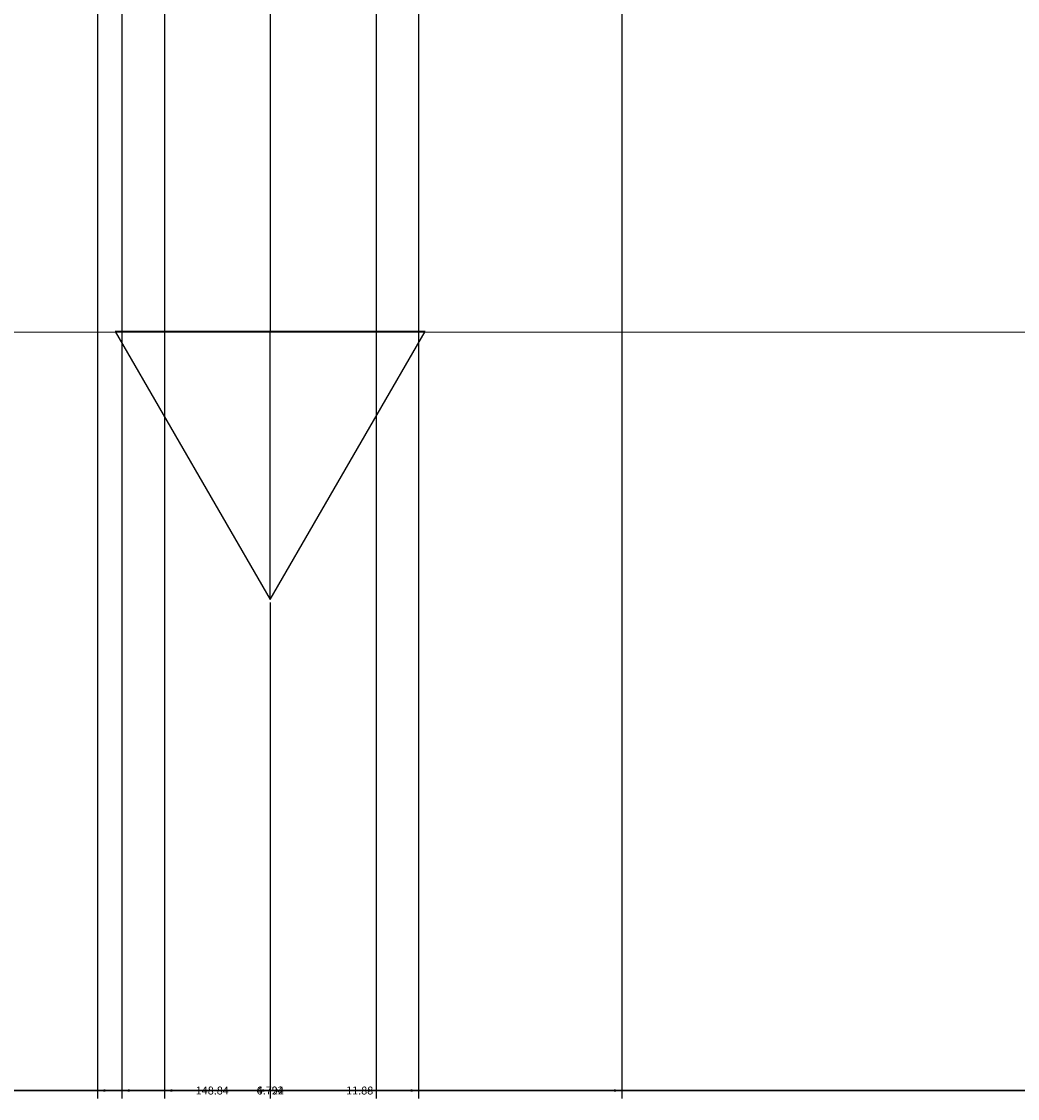
# Model space of a CAD drawing. Units: inches. Extents: x 412 to 584, y 208 to 437.
# Tile 6 of 28: x 494 to 516, y 208 to 233. Entities that reach past the tile are written whole.
import ezdxf

# ---------------------------------------------------------------- set-up
doc = ezdxf.new("R2010")
doc.units = ezdxf.units.IN
doc.header["$MEASUREMENT"] = 0
for name, color, linetype, lineweight in [('A-ANNO-DIMS', 2, 'Continuous', 18), ('E-ENCL', 8, 'Continuous', 18), ('E-POWR-EQPM', 3, 'Continuous', 25)]:
    doc.layers.add(name, color=color, linetype=linetype, lineweight=lineweight)
doc.styles.get("Standard").update_dxf_attribs({"font": 'arial.ttf'})
doc.dimstyles.get("Standard").update_dxf_attribs({"dimtxt": 0.18, "dimasz": 0.18, "dimexe": 0.18, "dimexo": 0.0625, "dimgap": 0.09, "dimtad": 0, "dimtih": 1, "dimtoh": 1, "dimdec": 4, "dimzin": 0, "dimdsep": 46, "dimtxsty": 'Standard', "dimcen": 0.09, "dimadec": 0, "dimazin": 0, "dimtfac": 1, "dimtdec": 4, "dimtofl": 0, "dimtmove": 0, "dimatfit": 3, "dimfxl": 1, "dimtolj": 1, "dimtzin": 0, "dimarcsym": 0})

# ---------------------------------------------------------------- blocks, each defined once
blk = doc.blocks.new('*U3')
blk.add_line((-0.212, 0.212), (0.212, -0.212))
blk = doc.blocks.new('*U4')
at = {"color": 0, "linetype": 'ByBlock', "lineweight": -2, "transparency": 16777216}
for p, rotation in [((224.254, 56.203), 180), ((224.677, 56.203), 89.99999999999999), ((224.254, 55.78), 269.9999999999999)]:
    blk.add_blockref('*U3', p, dxfattribs=dict(at, rotation=rotation))
blk.add_blockref('*U3', (224.677, 55.78), dxfattribs=at)
blk = doc.blocks.new('*U7')
blk.add_line((-0.288, 0.288), (0.288, -0.288))
blk = doc.blocks.new('*U8')
at = {"color": 0, "linetype": 'ByBlock', "lineweight": -2, "transparency": 16777216}
for p, rotation in [((224.177, 56.28), 180), ((224.754, 56.28), 90), ((224.177, 55.703), 269.9999999999999)]:
    blk.add_blockref('*U7', p, dxfattribs=dict(at, rotation=rotation))
blk.add_blockref('*U7', (224.754, 55.703), dxfattribs=at)
blk = doc.blocks.new('MCCB-800A')
for q in [(1.94, 18.628), (3.361, 0)]:
    blk.add_line((3.361, 14.893), q)
blk.add_lwpolyline([(0, 20.016), (6.722, 20.016), (6.722, 12.209), (0, 12.209)], close=True)
blk.add_circle((3.361, 14.5), 0.393)
for name in ['*U8', '*U4']:
    blk.add_blockref(name, (-221.104, -36.809))
blk = doc.blocks.new('*D13')
at = {"layer": 'A-ANNO-DIMS', "color": 0, "lineweight": -2, "transparency": 16777216}
for p, q in [((423.556, 225.526), (423.556, 208.233)), ((572.394, 225.526), (572.394, 208.233)), ((423.736, 208.413), (497.52, 208.413)), ((572.214, 208.413), (498.43, 208.413))]:
    blk.add_line(p, q, dxfattribs=at)
at = {"layer": 'A-ANNO-DIMS', "color": 0, "transparency": 16777216}
for points in [[(423.736, 208.443), (423.736, 208.383), (423.556, 208.413)], [(572.214, 208.443), (572.214, 208.383), (572.394, 208.413)]]:
    blk.add_solid(points, dxfattribs=at)
at = {"layer": 'Defpoints', "color": 0, "transparency": 16777216}
for p in [(423.556, 225.588), (572.394, 225.588), (572.394, 208.413)]:
    blk.add_point(p, dxfattribs=at)
at = {"layer": 'A-ANNO-DIMS', "color": 0, "transparency": 16777216, "insert": (497.975, 208.413), "char_height": 0.18, "attachment_point": 5}
blk.add_mtext('\\A1;148.84', dxfattribs=at)
blk = doc.blocks.new('*D15')
at = {"layer": 'A-ANNO-DIMS', "color": 0, "lineweight": -2, "transparency": 16777216}
for p, q in [((454.644, 219.451), (454.644, 208.233)), ((499.288, 219.47), (499.288, 208.233)), ((454.824, 208.413), (476.569, 208.413)), ((499.108, 208.413), (477.363, 208.413))]:
    blk.add_line(p, q, dxfattribs=at)
at = {"layer": 'A-ANNO-DIMS', "color": 0, "transparency": 16777216}
for points in [[(454.824, 208.443), (454.824, 208.383), (454.644, 208.413)], [(499.108, 208.443), (499.108, 208.383), (499.288, 208.413)]]:
    blk.add_solid(points, dxfattribs=at)
at = {"layer": 'Defpoints', "color": 0, "transparency": 16777216}
for p in [(454.644, 219.513), (499.288, 219.533), (499.288, 208.413)]:
    blk.add_point(p, dxfattribs=at)
at = {"layer": 'A-ANNO-DIMS', "color": 0, "transparency": 16777216, "insert": (476.966, 208.413), "char_height": 0.18, "attachment_point": 5}
blk.add_mtext('\\A1;44.64', dxfattribs=at)
blk = doc.blocks.new('*D16')
at = {"layer": 'A-ANNO-DIMS', "color": 0, "lineweight": -2, "transparency": 16777216}
for p, q in [((499.288, 219.47), (499.288, 208.233)), ((550.135, 219.451), (550.135, 208.233)), ((499.468, 208.413), (524.317, 208.413)), ((549.955, 208.413), (525.106, 208.413))]:
    blk.add_line(p, q, dxfattribs=at)
at = {"layer": 'A-ANNO-DIMS', "color": 0, "transparency": 16777216}
for points in [[(499.468, 208.443), (499.468, 208.383), (499.288, 208.413)], [(549.955, 208.443), (549.955, 208.383), (550.135, 208.413)]]:
    blk.add_solid(points, dxfattribs=at)
at = {"layer": 'Defpoints', "color": 0, "transparency": 16777216}
for p in [(499.288, 219.533), (550.135, 219.513), (550.135, 208.413)]:
    blk.add_point(p, dxfattribs=at)
at = {"layer": 'A-ANNO-DIMS', "color": 0, "transparency": 16777216, "insert": (524.711, 208.413), "char_height": 0.18, "attachment_point": 5}
blk.add_mtext('\\A1;50.85', dxfattribs=at)
blk = doc.blocks.new('*D17')
at = {"layer": 'A-ANNO-DIMS', "color": 0, "lineweight": -2, "transparency": 16777216}
for p, q in [((497.715, 426.185), (583.674, 426.185)), ((583.494, 426.005), (583.494, 323.031)), ((583.494, 219.693), (583.494, 322.667)), ((550.198, 219.513), (583.674, 219.513))]:
    blk.add_line(p, q, dxfattribs=at)
at = {"layer": 'A-ANNO-DIMS', "color": 0, "transparency": 16777216}
for points in [[(583.464, 426.005), (583.524, 426.005), (583.494, 426.185)], [(583.464, 219.693), (583.524, 219.693), (583.494, 219.513)]]:
    blk.add_solid(points, dxfattribs=at)
at = {"layer": 'Defpoints', "color": 0, "transparency": 16777216}
for p in [(497.652, 426.185), (550.135, 219.513), (583.494, 219.513)]:
    blk.add_point(p, dxfattribs=at)
at = {"layer": 'A-ANNO-DIMS', "color": 0, "transparency": 16777216, "insert": (583.494, 322.849), "char_height": 0.18, "attachment_point": 5}
blk.add_mtext('\\A1;206.67', dxfattribs=at)
blk = doc.blocks.new('*D29')
at = {"layer": 'A-ANNO-DIMS', "color": 0, "lineweight": -2, "transparency": 16777216}
for p, q in [((495.927, 378.924), (495.927, 208.233)), ((502.649, 378.924), (502.649, 208.233)), ((496.107, 208.413), (498.895, 208.413)), ((502.469, 208.413), (499.681, 208.413))]:
    blk.add_line(p, q, dxfattribs=at)
at = {"layer": 'A-ANNO-DIMS', "color": 0, "transparency": 16777216}
for points in [[(496.107, 208.443), (496.107, 208.383), (495.927, 208.413)], [(502.469, 208.443), (502.469, 208.383), (502.649, 208.413)]]:
    blk.add_solid(points, dxfattribs=at)
at = {"layer": 'Defpoints', "color": 0, "transparency": 16777216}
for p in [(495.927, 378.987), (502.649, 378.987), (502.649, 208.413)]:
    blk.add_point(p, dxfattribs=at)
at = {"layer": 'A-ANNO-DIMS', "color": 0, "transparency": 16777216, "insert": (499.288, 208.413), "char_height": 0.18, "attachment_point": 5}
blk.add_mtext('\\A1;6.722', dxfattribs=at)
blk = doc.blocks.new('*D31')
at = {"layer": 'A-ANNO-DIMS', "color": 0, "lineweight": -2, "transparency": 16777216}
for p, q in [((495.375, 405.385), (495.375, 208.233)), ((507.254, 405.385), (507.254, 208.233)), ((495.555, 208.413), (500.929, 208.413)), ((507.074, 208.413), (501.7, 208.413))]:
    blk.add_line(p, q, dxfattribs=at)
at = {"layer": 'A-ANNO-DIMS', "color": 0, "transparency": 16777216}
for points in [[(495.555, 208.443), (495.555, 208.383), (495.375, 208.413)], [(507.074, 208.443), (507.074, 208.383), (507.254, 208.413)]]:
    blk.add_solid(points, dxfattribs=at)
at = {"layer": 'Defpoints', "color": 0, "transparency": 16777216}
for p in [(495.375, 405.448), (507.254, 405.448), (507.254, 208.413)]:
    blk.add_point(p, dxfattribs=at)
at = {"layer": 'A-ANNO-DIMS', "color": 0, "transparency": 16777216, "insert": (501.314, 208.413), "char_height": 0.18, "attachment_point": 5}
blk.add_mtext('\\A1;11.88', dxfattribs=at)
blk = doc.blocks.new('*D39')
at = {"layer": 'A-ANNO-DIMS', "color": 0, "lineweight": -2, "transparency": 16777216}
for p, q in [((496.891, 346.914), (496.891, 208.233)), ((501.685, 346.914), (501.685, 208.233)), ((497.071, 208.413), (498.891, 208.413)), ((501.505, 208.413), (499.685, 208.413))]:
    blk.add_line(p, q, dxfattribs=at)
at = {"layer": 'A-ANNO-DIMS', "color": 0, "transparency": 16777216}
for points in [[(497.071, 208.443), (497.071, 208.383), (496.891, 208.413)], [(501.505, 208.443), (501.505, 208.383), (501.685, 208.413)]]:
    blk.add_solid(points, dxfattribs=at)
at = {"layer": 'Defpoints', "color": 0, "transparency": 16777216}
for p in [(496.891, 346.977), (501.685, 346.977), (501.685, 208.413)]:
    blk.add_point(p, dxfattribs=at)
at = {"layer": 'A-ANNO-DIMS', "color": 0, "transparency": 16777216, "insert": (499.288, 208.413), "char_height": 0.18, "attachment_point": 5}
blk.add_mtext('\\A1;4.794', dxfattribs=at)

msp = doc.modelspace()

# ---------------------------------------------------------------- linework, layer by layer
at = {"layer": 'E-ENCL'}
msp.add_lwpolyline([(423.5562, 309.3773), (572.3937, 309.3773), (572.3937, 225.5881), (423.5562, 225.5881)], close=True, dxfattribs=at)
at = {"layer": 'E-POWR-EQPM'}
msp.add_line((499.2878, 219.5329), (499.2878, 225.5881), dxfattribs=at)
msp.add_lwpolyline([(499.2878, 219.5329), (502.7952, 225.6078), (495.7805, 225.6078)], close=True, dxfattribs=at)

# ---------------------------------------------------------------- block references
msp.add_blockref('MCCB-800A', (495.9268, 225.6077), dxfattribs=at)

# ---------------------------------------------------------------- dimensions: what is measured, and where the dimension line sits
at = {"layer": 'A-ANNO-DIMS'}
dim = msp.add_linear_dim(base=(583.4937, 219.5133), p1=(497.6523, 426.1847), p2=(550.1351, 219.5133), angle=90, dimstyle='Standard', override={"dimdec": 2, "dimlfac": 1, "dimrnd": 0, "dimzin": 0, "dimdsep": 46, "dimlunit": 2}, dxfattribs=at)
dim.commit()
dim.dimension.update_dxf_attribs({"geometry": '*D17', "text_midpoint": (583.4937, 322.849)})
for base, p1, p2, override, picture, middle in [((507.2538, 208.4133), (495.3746, 405.448), (507.2538, 405.448), {"dimdec": 2, "dimlfac": 1, "dimrnd": 0, "dimzin": 0, "dimdsep": 46, "dimlunit": 2}, '*D31', (501.3142, 208.4133)), ((502.6489, 208.4133), (495.9268, 378.9867), (502.6489, 378.9867), {"dimdec": 3, "dimlfac": 1, "dimrnd": 0, "dimzin": 0, "dimdsep": 46, "dimlunit": 2}, '*D29', (499.2878, 208.4133)), ((501.6846, 208.4133), (496.891, 346.9765), (501.6846, 346.9765), {"dimdec": 3, "dimlfac": 1, "dimrnd": 0, "dimzin": 0, "dimdsep": 46, "dimlunit": 2}, '*D39', (499.2878, 208.4133)), ((572.3937, 208.4133), (423.5562, 225.5881), (572.3937, 225.5881), {"dimdec": 2, "dimlfac": 1, "dimrnd": 0, "dimzin": 0, "dimdsep": 46, "dimlunit": 2}, '*D13', (497.975, 208.4133)), ((499.2878, 208.4133), (454.6441, 219.5133), (499.2878, 219.5329), {"dimdec": 2, "dimlfac": 1, "dimrnd": 0, "dimzin": 0, "dimdsep": 46, "dimlunit": 2}, '*D15', (476.9659, 208.4133)), ((550.1351, 208.4133), (499.2878, 219.5329), (550.1351, 219.5133), {"dimdec": 2, "dimlfac": 1, "dimrnd": 0, "dimzin": 0, "dimdsep": 46, "dimlunit": 2}, '*D16', (524.7115, 208.4133))]:
    dim = msp.add_linear_dim(base=base, p1=p1, p2=p2, dimstyle='Standard', override=override, dxfattribs=at)
    dim.commit()
    dim.dimension.update_dxf_attribs({"geometry": picture, "text_midpoint": middle})

doc.saveas('drawing.dxf')
